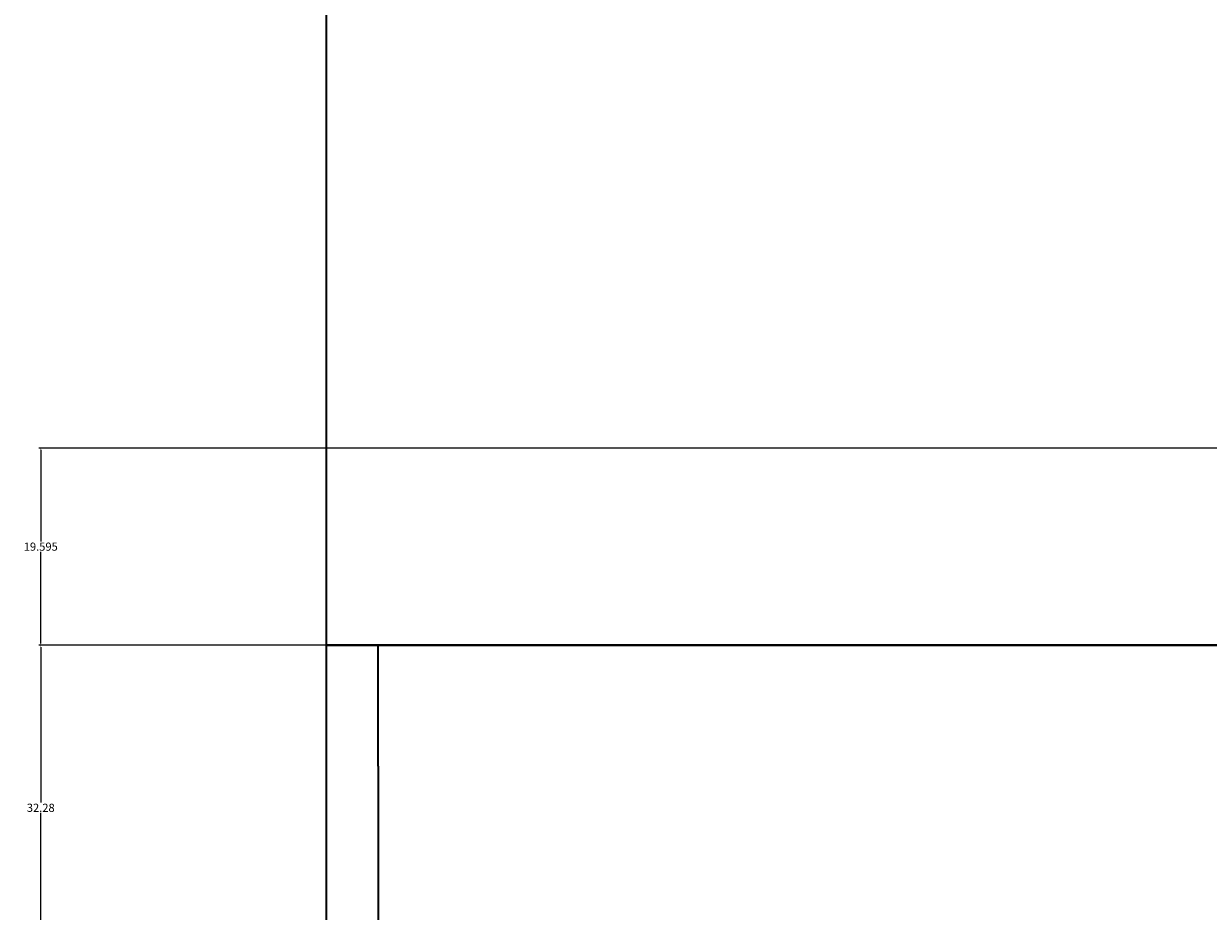
# Model space of a CAD drawing. Units: inches. Extents: x 69 to 650, y -16 to 573.
# Tile 11 of 26: x 69 to 187, y 218 to 306. Entities that reach past the tile are written whole.
import ezdxf

# ---------------------------------------------------------------- set-up
doc = ezdxf.new("R2010")
doc.units = ezdxf.units.IN
doc.header["$MEASUREMENT"] = 0
doc.layers.add('A-ANNO-DIMS', color=2, linetype='Continuous', lineweight=18)
doc.layers.add('A-WALL', color=7, linetype='Continuous', lineweight=35)
doc.styles.get("Standard").update_dxf_attribs({"font": 'arial.ttf'})
doc.dimstyles.get("Standard").update_dxf_attribs({"dimtxt": 0.8125, "dimasz": 0.18, "dimexe": 0.18, "dimexo": 0.0625, "dimgap": 0.09, "dimtad": 0, "dimtih": 1, "dimtoh": 1, "dimdec": 4, "dimzin": 0, "dimdsep": 46, "dimlunit": 4, "dimtxsty": 'Standard', "dimcen": 0.09, "dimadec": 0, "dimazin": 0, "dimtfac": 1, "dimtdec": 4, "dimtofl": 0, "dimtmove": 0, "dimatfit": 3, "dimfxl": 1, "dimtolj": 1, "dimtzin": 0, "dimarcsym": 0})

# ---------------------------------------------------------------- blocks, each defined once
blk = doc.blocks.new('*D19')
at = {"layer": 'A-ANNO-DIMS', "color": 0, "lineweight": -2, "transparency": 16777216}
for p, q in [((99.56, 471.72), (99.56, 572.74)), ((99.74, 572.56), (358.57, 572.56)), ((619.38, 572.56), (360.54, 572.56)), ((619.56, 87.99), (619.56, 572.74))]:
    blk.add_line(p, q, dxfattribs=at)
at = {"layer": 'A-ANNO-DIMS', "color": 0, "transparency": 16777216}
for points in [[(99.74, 572.59), (99.74, 572.53), (99.56, 572.56)], [(619.38, 572.59), (619.38, 572.53), (619.56, 572.56)]]:
    blk.add_solid(points, dxfattribs=at)
at = {"layer": 'Defpoints', "color": 0, "transparency": 16777216}
for p in [(619.56, 572.56), (99.56, 471.66), (619.56, 87.93)]:
    blk.add_point(p, dxfattribs=at)
at = {"layer": 'A-ANNO-DIMS', "color": 0, "transparency": 16777216, "insert": (359.56, 572.56), "char_height": 0.812, "attachment_point": 5}
blk.add_mtext('\\A1;520', dxfattribs=at)
blk = doc.blocks.new('*D25')
at = {"layer": 'A-ANNO-DIMS', "color": 0, "lineweight": -2, "transparency": 16777216}
for p, q in [((99.49, 243.93), (70.98, 243.93)), ((71.16, 243.75), (71.16, 228.3)), ((71.16, 211.83), (71.16, 227.29)), ((441.88, 211.65), (70.98, 211.65))]:
    blk.add_line(p, q, dxfattribs=at)
at = {"layer": 'A-ANNO-DIMS', "color": 0, "transparency": 16777216}
for points in [[(71.13, 243.75), (71.19, 243.75), (71.16, 243.93)], [(71.13, 211.83), (71.19, 211.83), (71.16, 211.65)]]:
    blk.add_solid(points, dxfattribs=at)
at = {"layer": 'Defpoints', "color": 0, "transparency": 16777216}
for p in [(71.16, 243.93), (99.56, 243.93), (441.94, 211.65)]:
    blk.add_point(p, dxfattribs=at)
at = {"layer": 'A-ANNO-DIMS', "color": 0, "transparency": 16777216, "insert": (71.16, 227.79), "char_height": 0.812, "attachment_point": 5}
blk.add_mtext('\\A1;32.28', dxfattribs=at)
blk = doc.blocks.new('*D35')
at = {"layer": 'A-ANNO-DIMS', "color": 0, "lineweight": -2, "transparency": 16777216}
for p, q in [((99.56, 243.87), (99.56, 35.35)), ((190.3, 243.87), (190.3, 35.35)), ((99.74, 35.53), (143.47, 35.53)), ((190.12, 35.53), (146.39, 35.53))]:
    blk.add_line(p, q, dxfattribs=at)
at = {"layer": 'A-ANNO-DIMS', "color": 0, "transparency": 16777216}
for points in [[(99.74, 35.56), (99.74, 35.5), (99.56, 35.53)], [(190.12, 35.56), (190.12, 35.5), (190.3, 35.53)]]:
    blk.add_solid(points, dxfattribs=at)
at = {"layer": 'Defpoints', "color": 0, "transparency": 16777216}
for p in [(99.56, 243.93), (190.3, 243.93), (190.3, 35.53)]:
    blk.add_point(p, dxfattribs=at)
at = {"layer": 'A-ANNO-DIMS', "color": 0, "transparency": 16777216, "insert": (144.93, 35.53), "char_height": 0.812, "attachment_point": 5}
blk.add_mtext('\\A1;90.74', dxfattribs=at)
blk = doc.blocks.new('*D58')
at = {"layer": 'A-ANNO-DIMS', "color": 0, "lineweight": -2, "transparency": 16777216}
for p, q in [((313.74, 263.53), (70.98, 263.53)), ((71.16, 263.35), (71.16, 254.23)), ((71.16, 244.11), (71.16, 253.22)), ((190.24, 243.93), (70.98, 243.93))]:
    blk.add_line(p, q, dxfattribs=at)
at = {"layer": 'A-ANNO-DIMS', "color": 0, "transparency": 16777216}
for points in [[(71.13, 263.35), (71.19, 263.35), (71.16, 263.53)], [(71.13, 244.11), (71.19, 244.11), (71.16, 243.93)]]:
    blk.add_solid(points, dxfattribs=at)
at = {"layer": 'Defpoints', "color": 0, "transparency": 16777216}
for p in [(71.16, 263.53), (313.81, 263.53), (190.3, 243.93)]:
    blk.add_point(p, dxfattribs=at)
at = {"layer": 'A-ANNO-DIMS', "color": 0, "transparency": 16777216, "insert": (71.16, 253.73), "char_height": 0.812, "attachment_point": 5}
blk.add_mtext('\\A1;19.595', dxfattribs=at)

msp = doc.modelspace()

# ---------------------------------------------------------------- linework, layer by layer
at = {"layer": 'A-WALL'}
for p, q in [((99.556, 243.93), (99.556, 411.93)), ((99.556, 243.93), (619.555, 243.93)), ((99.556, 231.93), (99.556, 243.93)), ((104.6982, 231.93), (104.6982, 243.93)), ((99.556, 87.93), (99.556, 231.93)), ((104.6982, 231.93), (104.6982, 87.93))]:
    msp.add_line(p, q, dxfattribs=at)
msp.add_lwpolyline([(99.556, 363.8739), (190.299, 363.8739), (190.299, 243.93), (99.556, 243.93)], close=True, dxfattribs=at)

# ---------------------------------------------------------------- dimensions: what is measured, and where the dimension line sits
at = {"layer": 'A-ANNO-DIMS'}
for base, p1, p2, override, picture, middle in [((619.555, 572.5573), (99.556, 471.6595), (619.555, 87.93), {"dimdec": 0, "dimlfac": 1, "dimrnd": 0, "dimzin": 0, "dimdsep": 46, "dimlunit": 2}, '*D19', (359.5555, 572.5573)), ((190.299, 35.53), (99.556, 243.93), (190.299, 243.93), {"dimdec": 2, "dimlfac": 1, "dimrnd": 0, "dimzin": 0, "dimdsep": 46, "dimlunit": 2}, '*D35', (144.9275, 35.53))]:
    dim = msp.add_linear_dim(base=base, p1=p1, p2=p2, dimstyle='Standard', override=override, dxfattribs=at)
    dim.commit()
    dim.dimension.update_dxf_attribs({"geometry": picture, "text_midpoint": middle})
for base, p1, p2, override, picture, middle in [((71.156, 263.5253), (190.299, 243.93), (313.8067, 263.5253), {"dimdec": 3, "dimlfac": 1, "dimrnd": 0, "dimzin": 0, "dimdsep": 46, "dimlunit": 2}, '*D58', (71.156, 253.7277)), ((71.156, 243.93), (441.9398, 211.6519), (99.556, 243.93), {"dimdec": 2, "dimlfac": 1, "dimrnd": 0, "dimzin": 0, "dimdsep": 46, "dimlunit": 2}, '*D25', (71.156, 227.7909))]:
    dim = msp.add_linear_dim(base=base, p1=p1, p2=p2, angle=90, dimstyle='Standard', override=override, dxfattribs=at)
    dim.commit()
    dim.dimension.update_dxf_attribs({"geometry": picture, "text_midpoint": middle})

doc.saveas('drawing.dxf')
